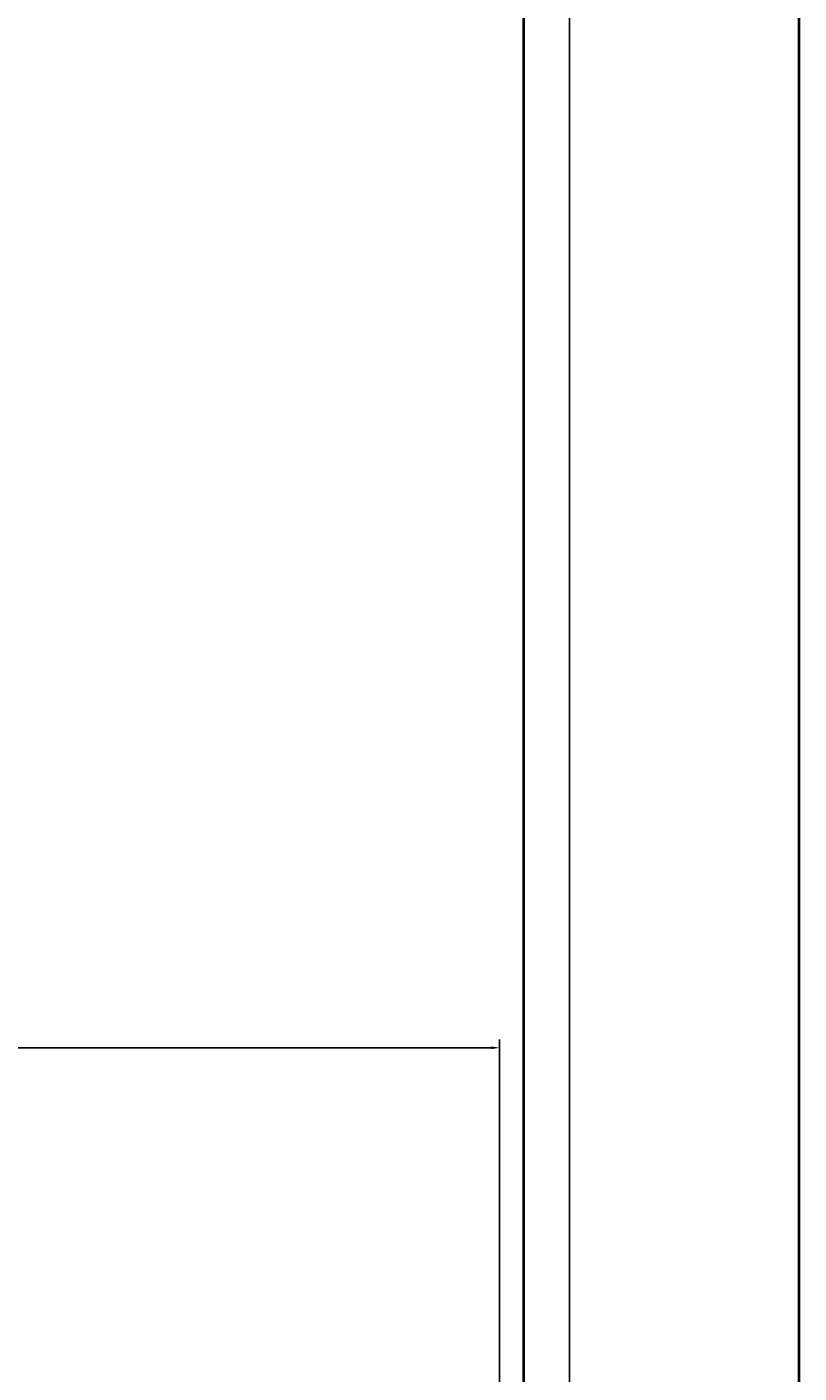
# Model space of a CAD drawing. Units: inches. Extents: x -301 to 715, y -607 to 364.
# Tile 82 of 141: x -62 to -46, y -39 to -10. Entities that reach past the tile are written whole.
import ezdxf

# ---------------------------------------------------------------- set-up
doc = ezdxf.new("R2010")
doc.units = ezdxf.units.IN
doc.header["$MEASUREMENT"] = 0
doc.layers.add('A-ANNO-DIMS', color=2, linetype='Continuous', lineweight=18)
doc.layers.add('A-WALL', color=3, linetype='Continuous', lineweight=40)
doc.styles.get("Standard").update_dxf_attribs({"font": 'arial.ttf'})
doc.dimstyles.get("Standard").update_dxf_attribs({"dimtxt": 0.18, "dimasz": 0.18, "dimexe": 0.18, "dimexo": 0.0625, "dimgap": 0.09, "dimtad": 0, "dimtih": 1, "dimtoh": 1, "dimdec": 1, "dimzin": 0, "dimdsep": 46, "dimlunit": 4, "dimtxsty": 'Standard', "dimcen": 0.09, "dimclrd": 3, "dimclre": 4, "dimclrt": 6, "dimadec": 0, "dimazin": 0, "dimtfac": 1, "dimtdec": 1, "dimtofl": 0, "dimtmove": 0, "dimatfit": 3, "dimfxl": 1, "dimtfill": 2, "dimtfillclr": 51, "dimtolj": 1, "dimtzin": 0, "dimarcsym": 0})

# ---------------------------------------------------------------- blocks, each defined once
blk = doc.blocks.new('*D114')
at = {"layer": 'A-ANNO-DIMS', "color": 4, "lineweight": -2, "transparency": 16777216}
for p, q in [((-103.477, -39.895), (-103.477, -32.076)), ((-52.128, -39.895), (-52.128, -32.076))]:
    blk.add_line(p, q, dxfattribs=at)
at = {"layer": 'A-ANNO-DIMS', "color": 3, "lineweight": -2, "transparency": 16777216}
for p, q in [((-103.297, -32.256), (-79.024, -32.256)), ((-52.308, -32.256), (-76.581, -32.256))]:
    blk.add_line(p, q, dxfattribs=at)
at = {"layer": 'A-ANNO-DIMS', "color": 3, "transparency": 16777216}
for points in [[(-103.297, -32.226), (-103.297, -32.286), (-103.477, -32.256)], [(-52.308, -32.226), (-52.308, -32.286), (-52.128, -32.256)]]:
    blk.add_solid(points, dxfattribs=at)
at = {"layer": 'Defpoints', "color": 0, "transparency": 16777216}
for p in [(-52.128, -32.256), (-103.477, -39.958), (-52.128, -39.958)]:
    blk.add_point(p, dxfattribs=at)
at = {"layer": 'A-ANNO-DIMS', "color": 6, "transparency": 16777216, "insert": (-77.803, -32.256), "char_height": 0.18, "attachment_point": 5, "bg_fill": 1, "box_fill_scale": 1.25, "bg_fill_color": 51, "bg_fill_transparency": 0}
blk.add_mtext('\\A1;DESK 4\'-3 1/2" TYP.', dxfattribs=at)
blk = doc.blocks.new('*D151')
at = {"layer": 'A-ANNO-DIMS', "color": 4, "lineweight": -2, "transparency": 16777216}
for p, q in [((-204.603, -223.755), (-204.603, 359.612)), ((-45.603, -214.755), (-45.603, 359.612))]:
    blk.add_line(p, q, dxfattribs=at)
at = {"layer": 'A-ANNO-DIMS', "color": 3, "lineweight": -2, "transparency": 16777216}
for p, q in [((-204.423, 359.432), (-125.494, 359.432)), ((-45.783, 359.432), (-124.713, 359.432))]:
    blk.add_line(p, q, dxfattribs=at)
at = {"layer": 'A-ANNO-DIMS', "color": 3, "transparency": 16777216}
for points in [[(-204.423, 359.462), (-204.423, 359.402), (-204.603, 359.432)], [(-45.783, 359.462), (-45.783, 359.402), (-45.603, 359.432)]]:
    blk.add_solid(points, dxfattribs=at)
at = {"layer": 'Defpoints', "color": 0, "transparency": 16777216}
for p in [(-45.603, 359.432), (-45.603, -214.818), (-204.603, -223.818)]:
    blk.add_point(p, dxfattribs=at)
at = {"layer": 'A-ANNO-DIMS', "color": 6, "transparency": 16777216, "insert": (-125.103, 359.432), "char_height": 0.18, "attachment_point": 5, "bg_fill": 1, "box_fill_scale": 1.25, "bg_fill_color": 51, "bg_fill_transparency": 0}
blk.add_mtext('\\A1;13\'-3"', dxfattribs=at)
blk = doc.blocks.new('*D158')
at = {"layer": 'A-ANNO-DIMS', "color": 4, "lineweight": -2, "transparency": 16777216}
for p, q in [((-122.603, 221.62), (-122.603, -296.865)), ((-50.603, 221.62), (-50.603, -296.865))]:
    blk.add_line(p, q, dxfattribs=at)
at = {"layer": 'A-ANNO-DIMS', "color": 3, "lineweight": -2, "transparency": 16777216}
for p, q in [((-122.423, -296.685), (-86.933, -296.685)), ((-50.783, -296.685), (-86.274, -296.685))]:
    blk.add_line(p, q, dxfattribs=at)
at = {"layer": 'A-ANNO-DIMS', "color": 3, "transparency": 16777216}
for points in [[(-122.423, -296.655), (-122.423, -296.715), (-122.603, -296.685)], [(-50.783, -296.655), (-50.783, -296.715), (-50.603, -296.685)]]:
    blk.add_solid(points, dxfattribs=at)
at = {"layer": 'Defpoints', "color": 0, "transparency": 16777216}
for p in [(-122.603, 221.682), (-50.603, 221.682), (-50.603, -296.685)]:
    blk.add_point(p, dxfattribs=at)
at = {"layer": 'A-ANNO-DIMS', "color": 6, "transparency": 16777216, "insert": (-86.603, -296.685), "char_height": 0.18, "attachment_point": 5, "bg_fill": 1, "box_fill_scale": 1.25, "bg_fill_color": 51, "bg_fill_transparency": 0}
blk.add_mtext('\\A1;6\'-0"', dxfattribs=at)

msp = doc.modelspace()

# ---------------------------------------------------------------- linework, layer by layer
at = {"layer": 'A-WALL'}
for p, q in [((-51.603, -67.318), (-51.603, 25.682)), ((-45.603, -73.318), (-45.603, 25.682))]:
    msp.add_line(p, q, dxfattribs=at)

# ---------------------------------------------------------------- dimensions: what is measured, and where the dimension line sits
at = {"layer": 'A-ANNO-DIMS'}
for base, p1, p2, picture, middle in [((-45.603, 359.432), (-204.603, -223.818), (-45.603, -214.818), '*D151', (-125.103, 359.432)), ((-50.603, -296.685), (-122.603, 221.682), (-50.603, 221.682), '*D158', (-86.603, -296.685))]:
    dim = msp.add_linear_dim(base=base, p1=p1, p2=p2, dimstyle='Standard', override={"dimdec": 1, "dimlfac": 1, "dimrnd": 0, "dimzin": 1, "dimdsep": 46, "dimlunit": 4, "dimfrac": 2}, dxfattribs=at)
    dim.commit()
    dim.dimension.update_dxf_attribs({"geometry": picture, "text_midpoint": middle})
dim = msp.add_linear_dim(base=(-52.128, -32.256), p1=(-103.477, -39.958), p2=(-52.128, -39.958), text='DESK <> TYP.', dimstyle='Standard', override={"dimdec": 1, "dimlfac": 1, "dimrnd": 0, "dimzin": 1, "dimdsep": 46, "dimlunit": 4, "dimfrac": 2}, dxfattribs=at)
dim.commit()
dim.dimension.update_dxf_attribs({"geometry": '*D114', "text_midpoint": (-77.803, -32.256)})

doc.saveas('drawing.dxf')
